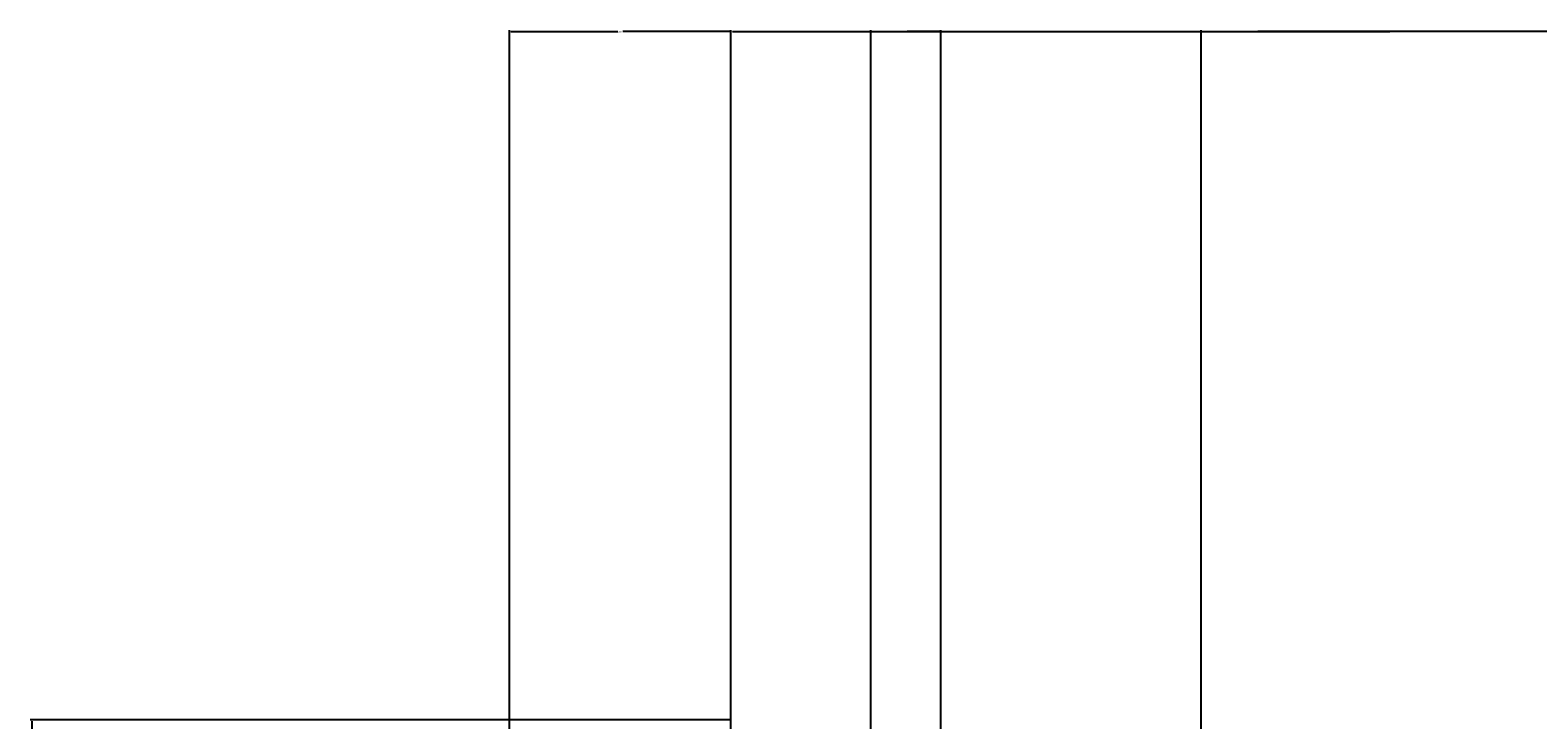
# Model space of a CAD drawing. Units: inches. Extents: x 1998 to 2588, y 1139 to 1977.
# Tile 75 of 134: x 1998 to 2192, y 1889 to 1977. Entities that reach past the tile are written whole.
import ezdxf

# ---------------------------------------------------------------- set-up
doc = ezdxf.new("R2010")
doc.units = ezdxf.units.IN
doc.layers.add('A-ANNO-DIMS', color=2, linetype='Continuous', lineweight=18)
doc.styles.get("Standard").update_dxf_attribs({"font": 'arial.ttf'})
doc.dimstyles.get("Standard").update_dxf_attribs({"dimtxt": 0.18, "dimasz": 0.18, "dimexe": 0.18, "dimexo": 0.0625, "dimgap": 0.09, "dimtad": 0, "dimtih": 1, "dimtoh": 1, "dimdec": 4, "dimzin": 0, "dimdsep": 46, "dimtxsty": 'Standard', "dimcen": 0.09, "dimadec": 0, "dimazin": 0, "dimtfac": 1, "dimtdec": 4, "dimtofl": 0, "dimtmove": 0, "dimatfit": 3, "dimfxl": 1, "dimtolj": 1, "dimtzin": 0, "dimarcsym": 0})

# ---------------------------------------------------------------- blocks, each defined once
blk = doc.blocks.new('*D25')
at = {"layer": 'A-ANNO-DIMS', "color": 0, "lineweight": -2, "transparency": 16777216}
for p, q in [((2087.97, 1888.79), (2087.97, 1977.36)), ((2088.15, 1977.18), (2155.19, 1977.18)), ((2222.79, 1977.18), (2155.75, 1977.18)), ((2222.97, 1888.79), (2222.97, 1977.36))]:
    blk.add_line(p, q, dxfattribs=at)
at = {"layer": 'A-ANNO-DIMS', "color": 0, "transparency": 16777216}
for points in [[(2088.15, 1977.21), (2088.15, 1977.15), (2087.97, 1977.18)], [(2222.79, 1977.21), (2222.79, 1977.15), (2222.97, 1977.18)]]:
    blk.add_solid(points, dxfattribs=at)
at = {"layer": 'Defpoints', "color": 0, "transparency": 16777216}
for p in [(2222.97, 1977.18), (2087.97, 1888.73), (2222.97, 1888.73)]:
    blk.add_point(p, dxfattribs=at)
at = {"layer": 'A-ANNO-DIMS', "color": 0, "transparency": 16777216, "insert": (2155.47, 1977.18), "char_height": 0.18, "attachment_point": 5}
blk.add_mtext('\\A1;135', dxfattribs=at)
blk = doc.blocks.new('*D28')
at = {"layer": 'A-ANNO-DIMS', "color": 0, "lineweight": -2, "transparency": 16777216}
for p, q in [((2059.47, 1759.79), (2059.47, 1977.36)), ((2059.65, 1977.18), (2073.4, 1977.18)), ((2087.79, 1977.18), (2074.05, 1977.18)), ((2087.97, 1759.79), (2087.97, 1977.36))]:
    blk.add_line(p, q, dxfattribs=at)
at = {"layer": 'A-ANNO-DIMS', "color": 0, "transparency": 16777216}
for points in [[(2059.65, 1977.21), (2059.65, 1977.15), (2059.47, 1977.18)], [(2087.79, 1977.21), (2087.79, 1977.15), (2087.97, 1977.18)]]:
    blk.add_solid(points, dxfattribs=at)
at = {"layer": 'Defpoints', "color": 0, "transparency": 16777216}
for p in [(2087.97, 1977.18), (2059.47, 1759.73), (2087.97, 1759.73)]:
    blk.add_point(p, dxfattribs=at)
at = {"layer": 'A-ANNO-DIMS', "color": 0, "transparency": 16777216, "insert": (2073.72, 1977.18), "char_height": 0.18, "attachment_point": 5}
blk.add_mtext('\\A1;28.5', dxfattribs=at)
blk = doc.blocks.new('*D29')
at = {"layer": 'A-ANNO-DIMS', "color": 0, "lineweight": -2, "transparency": 16777216}
for p, q in [((2087.91, 1888.73), (1997.84, 1888.73)), ((1998.02, 1888.55), (1998.02, 1824.41)), ((1998.02, 1759.91), (1998.02, 1824.05)), ((2059.41, 1759.73), (1997.84, 1759.73))]:
    blk.add_line(p, q, dxfattribs=at)
at = {"layer": 'A-ANNO-DIMS', "color": 0, "transparency": 16777216}
for points in [[(1997.99, 1888.55), (1998.05, 1888.55), (1998.02, 1888.73)], [(1997.99, 1759.91), (1998.05, 1759.91), (1998.02, 1759.73)]]:
    blk.add_solid(points, dxfattribs=at)
at = {"layer": 'Defpoints', "color": 0, "transparency": 16777216}
for p in [(1998.02, 1888.73), (2087.97, 1888.73), (2059.47, 1759.73)]:
    blk.add_point(p, dxfattribs=at)
at = {"layer": 'A-ANNO-DIMS', "color": 0, "transparency": 16777216, "insert": (1998.02, 1824.23), "char_height": 0.18, "attachment_point": 5}
blk.add_mtext('\\A1;129', dxfattribs=at)
blk = doc.blocks.new('*D37')
at = {"layer": 'A-ANNO-DIMS', "color": 0, "lineweight": -2, "transparency": 16777216}
for p, q in [((2148.45, 1612.79), (2148.45, 1977.36)), ((2148.63, 1977.18), (2172.73, 1977.18)), ((2197.27, 1977.18), (2173.18, 1977.18)), ((2197.45, 1612.79), (2197.45, 1977.36))]:
    blk.add_line(p, q, dxfattribs=at)
at = {"layer": 'A-ANNO-DIMS', "color": 0, "transparency": 16777216}
for points in [[(2148.63, 1977.21), (2148.63, 1977.15), (2148.45, 1977.18)], [(2197.27, 1977.21), (2197.27, 1977.15), (2197.45, 1977.18)]]:
    blk.add_solid(points, dxfattribs=at)
at = {"layer": 'Defpoints', "color": 0, "transparency": 16777216}
for p in [(2197.45, 1977.18), (2148.45, 1612.73), (2197.45, 1612.73)]:
    blk.add_point(p, dxfattribs=at)
at = {"layer": 'A-ANNO-DIMS', "color": 0, "transparency": 16777216, "insert": (2172.95, 1977.18), "char_height": 0.18, "attachment_point": 5}
blk.add_mtext('\\A1;49', dxfattribs=at)
blk = doc.blocks.new('*D40')
at = {"layer": 'A-ANNO-DIMS', "color": 0, "lineweight": -2, "transparency": 16777216}
for p, q in [((2105.97, 1628.54), (2105.97, 1977.36)), ((2106.15, 1977.18), (2110.32, 1977.18)), ((2114.79, 1977.18), (2110.62, 1977.18)), ((2114.97, 1628.8), (2114.97, 1977.36))]:
    blk.add_line(p, q, dxfattribs=at)
at = {"layer": 'A-ANNO-DIMS', "color": 0, "transparency": 16777216}
for points in [[(2106.15, 1977.21), (2106.15, 1977.15), (2105.97, 1977.18)], [(2114.79, 1977.21), (2114.79, 1977.15), (2114.97, 1977.18)]]:
    blk.add_solid(points, dxfattribs=at)
at = {"layer": 'Defpoints', "color": 0, "transparency": 16777216}
for p in [(2114.97, 1977.18), (2105.97, 1628.48), (2114.97, 1628.74)]:
    blk.add_point(p, dxfattribs=at)
at = {"layer": 'A-ANNO-DIMS', "color": 0, "transparency": 16777216, "insert": (2110.47, 1977.18), "char_height": 0.18, "attachment_point": 5}
blk.add_mtext('\\A1;9', dxfattribs=at)

msp = doc.modelspace()

# ---------------------------------------------------------------- dimensions: what is measured, and where the dimension line sits
at = {"layer": 'A-ANNO-DIMS'}
for base, p1, p2, override, picture, middle in [((2087.9729, 1977.1824), (2059.4729, 1759.7324), (2087.9729, 1759.7324), {"dimdec": 1, "dimlfac": 1, "dimrnd": 0, "dimzin": 0, "dimdsep": 46, "dimlunit": 2}, '*D28', (2073.7229, 1977.1824)), ((2222.9729, 1977.1824), (2087.9729, 1888.7324), (2222.9729, 1888.7324), {"dimdec": 0, "dimlfac": 1, "dimrnd": 0, "dimzin": 0, "dimdsep": 46, "dimlunit": 2}, '*D25', (2155.4729, 1977.1824)), ((2114.9729, 1977.1824), (2105.9729, 1628.4781), (2114.9729, 1628.7416), {"dimdec": 0, "dimlfac": 1, "dimrnd": 0, "dimzin": 0, "dimdsep": 46, "dimlunit": 2}, '*D40', (2110.4729, 1977.1824)), ((2197.4499, 1977.1824), (2148.4548, 1612.7324), (2197.4499, 1612.7324), {"dimdec": 0, "dimlfac": 1, "dimrnd": 0, "dimzin": 0, "dimdsep": 46, "dimlunit": 2}, '*D37', (2172.9524, 1977.1824))]:
    dim = msp.add_linear_dim(base=base, p1=p1, p2=p2, dimstyle='Standard', override=override, dxfattribs=at)
    dim.commit()
    dim.dimension.update_dxf_attribs({"geometry": picture, "text_midpoint": middle})
dim = msp.add_linear_dim(base=(1998.0229, 1888.7324), p1=(2059.4729, 1759.7324), p2=(2087.9729, 1888.7324), angle=90, dimstyle='Standard', override={"dimdec": 0, "dimlfac": 1, "dimrnd": 0, "dimzin": 0, "dimdsep": 46, "dimlunit": 2}, dxfattribs=at)
dim.commit()
dim.dimension.update_dxf_attribs({"geometry": '*D29', "text_midpoint": (1998.0229, 1824.2324)})

doc.saveas('drawing.dxf')
